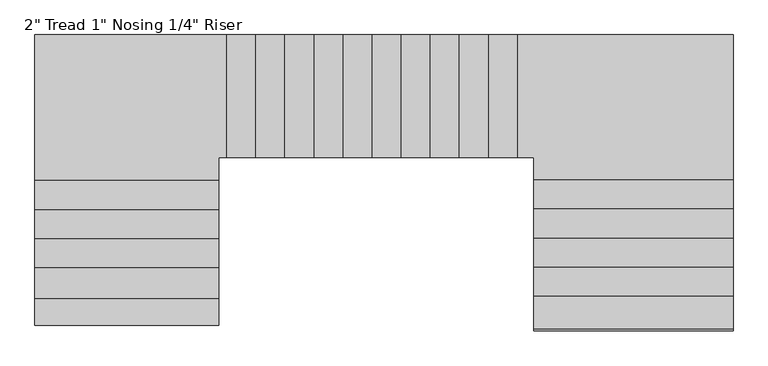
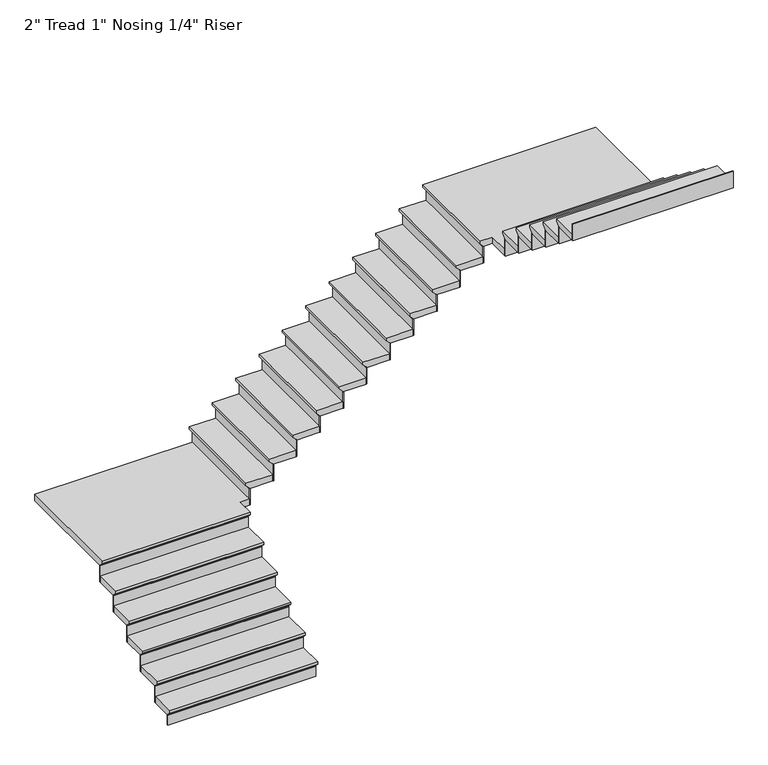
"""IFC4 building model written with IfcOpenShell, lengths in millimetres: stair flight geometry."""

from ifc_helpers import new_model, si_unit, origin, place, context, project, spatial, faceted_brep, source, transform, mapped, element, save


def stair_flight_3cceab32(model_context):
    return source(origin(), model_context, "Body", "Brep", [
        faceted_brep([(-2368.6972892, 4718.9167606, 6514.2717391), (-2368.6972892, 4718.9167606, 6533.3217391), (-3493.0046642, 4718.9167606, 6533.3217391), (-3493.0046642, 4718.9167606, 6514.2717391), (-2368.6972892, 4744.3167606, 6488.8717391), (-3493.0046642, 4744.3167606, 6488.8717391), (-2368.6972892, 4909.4167606, 6533.3217391), (-3493.0046642, 4909.4167606, 6533.3217391), (-3493.0046642, 4744.3167606, 6482.5217391), (-3493.0046642, 4909.4167606, 6482.5217391), (-2368.6972892, 4909.4167606, 6482.5217391), (-2368.6972892, 4744.3167606, 6482.5217391)], [[[0, 1, 2, 3]], [[4, 0, 3, 5]], [[2, 1, 6, 7]], [[8, 9, 10, 11]], [[2, 7, 9, 8, 5, 3]], [[8, 11, 4, 5]], [[6, 1, 0, 4, 11, 10]], [[7, 6, 10, 9]]]),
        faceted_brep([(-2368.6972892, 4744.3167606, 6482.5217391), (-2368.6972892, 4744.3167606, 6400.8), (-2368.6972892, 4750.6667606, 6400.8), (-2368.6972892, 4750.6667606, 6482.5217391), (-3493.0046642, 4744.3167606, 6482.5217391), (-3493.0046642, 4750.6667606, 6482.5217391), (-3493.0046642, 4750.6667606, 6400.8), (-3493.0046642, 4744.3167606, 6400.8)], [[[0, 1, 2, 3]], [[4, 5, 6, 7]], [[1, 0, 4, 7]], [[2, 1, 7, 6]], [[3, 2, 6, 5]], [[0, 3, 5, 4]]]),
        faceted_brep([(-2368.6972892, 4909.4167606, 6615.0434783), (-2368.6972892, 4909.4167606, 6482.5217391), (-2368.6972892, 4915.7667606, 6482.5217391), (-2368.6972892, 4915.7667606, 6615.0434783), (-3493.0046642, 4909.4167606, 6615.0434783), (-3493.0046642, 4915.7667606, 6615.0434783), (-3493.0046642, 4915.7667606, 6482.5217391), (-3493.0046642, 4909.4167606, 6482.5217391)], [[[0, 1, 2, 3]], [[4, 5, 6, 7]], [[1, 0, 4, 7]], [[2, 1, 7, 6]], [[3, 2, 6, 5]], [[0, 3, 5, 4]]]),
        faceted_brep([(-3493.0046642, 4884.0167606, 6665.8434783), (-2368.6972892, 4884.0167606, 6665.8434783), (-2368.6972892, 5099.9164494, 6665.8434783), (-3493.0046642, 5099.9164494, 6665.8434783), (-3493.0046642, 4909.4167606, 6615.0434783), (-3493.0046642, 5099.9164494, 6615.0434783), (-2368.6972892, 5099.9164494, 6615.0434783), (-2368.6972892, 4909.4167606, 6615.0434783), (-3493.0046642, 4909.4167606, 6621.3934783), (-3493.0046642, 4884.0167606, 6646.7934783), (-2368.6972892, 4909.4167606, 6621.3934783), (-2368.6972892, 4884.0167606, 6646.7934783)], [[[0, 1, 2, 3]], [[4, 5, 6, 7]], [[0, 3, 5, 4, 8, 9]], [[4, 7, 10, 8]], [[2, 1, 11, 10, 7, 6]], [[3, 2, 6, 5]], [[11, 1, 0, 9]], [[10, 11, 9, 8]]]),
        faceted_brep([(-2368.6972892, 5099.9164494, 6747.5652174), (-2368.6972892, 5099.9164494, 6615.0434783), (-2368.6972892, 5106.2664494, 6615.0434783), (-2368.6972892, 5106.2664494, 6747.5652174), (-3493.0046642, 5099.9164494, 6747.5652174), (-3493.0046642, 5106.2664494, 6747.5652174), (-3493.0046642, 5106.2664494, 6615.0434783), (-3493.0046642, 5099.9164494, 6615.0434783)], [[[0, 1, 2, 3]], [[4, 5, 6, 7]], [[1, 0, 4, 7]], [[2, 1, 7, 6]], [[3, 2, 6, 5]], [[0, 3, 5, 4]]]),
        faceted_brep([(-3493.0046642, 5074.5164494, 6798.3652174), (-2368.6972892, 5074.5164494, 6798.3652174), (-2368.6972892, 5277.7164494, 6798.3652174), (-3493.0046642, 5277.7164494, 6798.3652174), (-3493.0046642, 5099.9164494, 6747.5652174), (-3493.0046642, 5277.7164494, 6747.5652174), (-2368.6972892, 5277.7164494, 6747.5652174), (-2368.6972892, 5099.9164494, 6747.5652174), (-3493.0046642, 5099.9164494, 6753.9152174), (-3493.0046642, 5074.5164494, 6779.3152174), (-2368.6972892, 5099.9164494, 6753.9152174), (-2368.6972892, 5074.5164494, 6779.3152174)], [[[0, 1, 2, 3]], [[4, 5, 6, 7]], [[0, 3, 5, 4, 8, 9]], [[4, 7, 10, 8]], [[2, 1, 11, 10, 7, 6]], [[3, 2, 6, 5]], [[11, 1, 0, 9]], [[10, 11, 9, 8]]]),
        faceted_brep([(-2368.6972892, 5277.7164494, 6880.0869565), (-2368.6972892, 5277.7164494, 6747.5652174), (-2368.6972892, 5284.0664494, 6747.5652174), (-2368.6972892, 5284.0664494, 6880.0869565), (-3493.0046642, 5277.7164494, 6880.0869565), (-3493.0046642, 5284.0664494, 6880.0869565), (-3493.0046642, 5284.0664494, 6747.5652174), (-3493.0046642, 5277.7164494, 6747.5652174)], [[[0, 1, 2, 3]], [[4, 5, 6, 7]], [[1, 0, 4, 7]], [[2, 1, 7, 6]], [[3, 2, 6, 5]], [[0, 3, 5, 4]]]),
        faceted_brep([(-3493.0046642, 5252.3164494, 6930.8869565), (-2368.6972892, 5252.3164494, 6930.8869565), (-2368.6972892, 5455.5164494, 6930.8869565), (-3493.0046642, 5455.5164494, 6930.8869565), (-3493.0046642, 5277.7164494, 6880.0869565), (-3493.0046642, 5455.5164494, 6880.0869565), (-2368.6972892, 5455.5164494, 6880.0869565), (-2368.6972892, 5277.7164494, 6880.0869565), (-3493.0046642, 5277.7164494, 6886.4369565), (-3493.0046642, 5252.3164494, 6911.8369565), (-2368.6972892, 5277.7164494, 6886.4369565), (-2368.6972892, 5252.3164494, 6911.8369565)], [[[0, 1, 2, 3]], [[4, 5, 6, 7]], [[0, 3, 5, 4, 8, 9]], [[4, 7, 10, 8]], [[2, 1, 11, 10, 7, 6]], [[3, 2, 6, 5]], [[11, 1, 0, 9]], [[10, 11, 9, 8]]]),
        faceted_brep([(-2368.6972892, 5455.5164494, 7012.6086957), (-2368.6972892, 5455.5164494, 6880.0869565), (-2368.6972892, 5461.8664494, 6880.0869565), (-2368.6972892, 5461.8664494, 7012.6086957), (-3493.0046642, 5455.5164494, 7012.6086957), (-3493.0046642, 5461.8664494, 7012.6086957), (-3493.0046642, 5461.8664494, 6880.0869565), (-3493.0046642, 5455.5164494, 6880.0869565)], [[[0, 1, 2, 3]], [[4, 5, 6, 7]], [[1, 0, 4, 7]], [[2, 1, 7, 6]], [[3, 2, 6, 5]], [[0, 3, 5, 4]]]),
        faceted_brep([(-3493.0046642, 5430.1164494, 7063.4086957), (-2368.6972892, 5430.1164494, 7063.4086957), (-2368.6972892, 5633.3167606, 7063.4086957), (-3493.0046642, 5633.3167606, 7063.4086957), (-3493.0046642, 5455.5164494, 7012.6086957), (-3493.0046642, 5633.3167606, 7012.6086957), (-2368.6972892, 5633.3167606, 7012.6086957), (-2368.6972892, 5455.5164494, 7012.6086957), (-3493.0046642, 5455.5164494, 7018.9586957), (-3493.0046642, 5430.1164494, 7044.3586957), (-2368.6972892, 5455.5164494, 7018.9586957), (-2368.6972892, 5430.1164494, 7044.3586957)], [[[0, 1, 2, 3]], [[4, 5, 6, 7]], [[0, 3, 5, 4, 8, 9]], [[4, 7, 10, 8]], [[2, 1, 11, 10, 7, 6]], [[3, 2, 6, 5]], [[11, 1, 0, 9]], [[10, 11, 9, 8]]]),
        faceted_brep([(-2368.6972892, 5633.3167606, 7145.1304348), (-2368.6972892, 5633.3167606, 7012.6086957), (-2368.6972892, 5639.6667606, 7012.6086957), (-2368.6972892, 5639.6667606, 7145.1304348), (-3493.0046642, 5633.3167606, 7145.1304348), (-3493.0046642, 5639.6667606, 7145.1304348), (-3493.0046642, 5639.6667606, 7012.6086957), (-3493.0046642, 5633.3167606, 7012.6086957)], [[[0, 1, 2, 3]], [[4, 5, 6, 7]], [[1, 0, 4, 7]], [[2, 1, 7, 6]], [[3, 2, 6, 5]], [[0, 3, 5, 4]]]),
        faceted_brep([(-2295.032382, 6496.9167606, 7195.9304348), (-3493.0046642, 6496.9167606, 7195.9304348), (-3493.0046642, 5607.9167606, 7195.9304348), (-2368.6972892, 5607.9167606, 7195.9304348), (-2368.6972892, 5746.5536537, 7195.9304348), (-2295.032382, 5746.5536537, 7195.9304348), (-3493.0046642, 6496.9167606, 7145.1304348), (-2295.032382, 6496.9167606, 7145.1304348), (-2295.032382, 5746.5536537, 7145.1304348), (-2368.6972892, 5746.5536537, 7145.1304348), (-2368.6972892, 5633.3167606, 7145.1304348), (-3493.0046642, 5633.3167606, 7145.1304348), (-3493.0046642, 5633.3167606, 7151.4804348), (-3493.0046642, 5607.9167606, 7176.8804348), (-2368.6972892, 5633.3167606, 7151.4804348), (-2368.6972892, 5607.9167606, 7176.8804348)], [[[0, 1, 2, 3, 4, 5]], [[6, 7, 8, 9, 10, 11]], [[1, 0, 7, 6]], [[2, 1, 6, 11, 12, 13]], [[11, 10, 14, 12]], [[4, 3, 15, 14, 10, 9]], [[5, 4, 9, 8]], [[0, 5, 8, 7]], [[15, 3, 2, 13]], [[14, 15, 13, 12]]]),
        faceted_brep([(-2295.032382, 5746.5536537, 7277.6521739), (-2295.032382, 5746.5536537, 7145.1304348), (-2288.682382, 5746.5536537, 7145.1304348), (-2288.682382, 5746.5536537, 7277.6521739), (-2295.032382, 6496.9167606, 7277.6521739), (-2288.682382, 6496.9167606, 7277.6521739), (-2288.682382, 6496.9167606, 7145.1304348), (-2295.032382, 6496.9167606, 7145.1304348)], [[[0, 1, 2, 3]], [[4, 5, 6, 7]], [[1, 0, 4, 7]], [[2, 1, 7, 6]], [[3, 2, 6, 5]], [[0, 3, 5, 4]]]),
        faceted_brep([(-2320.432382, 6496.9167606, 7328.4521739), (-2320.432382, 5746.5536537, 7328.4521739), (-2117.232382, 5746.5536537, 7328.4521739), (-2117.232382, 6496.9167606, 7328.4521739), (-2295.032382, 6496.9167606, 7277.6521739), (-2117.232382, 6496.9167606, 7277.6521739), (-2117.232382, 5746.5536537, 7277.6521739), (-2295.032382, 5746.5536537, 7277.6521739), (-2295.032382, 6496.9167606, 7284.0021739), (-2320.432382, 6496.9167606, 7309.4021739), (-2295.032382, 5746.5536537, 7284.0021739), (-2320.432382, 5746.5536537, 7309.4021739)], [[[0, 1, 2, 3]], [[4, 5, 6, 7]], [[0, 3, 5, 4, 8, 9]], [[4, 7, 10, 8]], [[2, 1, 11, 10, 7, 6]], [[3, 2, 6, 5]], [[11, 1, 0, 9]], [[10, 11, 9, 8]]]),
        faceted_brep([(-2117.232382, 5746.5536537, 7410.173913), (-2117.232382, 5746.5536537, 7277.6521739), (-2110.882382, 5746.5536537, 7277.6521739), (-2110.882382, 5746.5536537, 7410.173913), (-2117.232382, 6496.9167606, 7410.173913), (-2110.882382, 6496.9167606, 7410.173913), (-2110.882382, 6496.9167606, 7277.6521739), (-2117.232382, 6496.9167606, 7277.6521739)], [[[0, 1, 2, 3]], [[4, 5, 6, 7]], [[1, 0, 4, 7]], [[2, 1, 7, 6]], [[3, 2, 6, 5]], [[0, 3, 5, 4]]]),
        faceted_brep([(-2142.632382, 6496.9167606, 7460.973913), (-2142.632382, 5746.5536537, 7460.973913), (-1939.432382, 5746.5536537, 7460.973913), (-1939.432382, 6496.9167606, 7460.973913), (-2117.232382, 6496.9167606, 7410.173913), (-1939.432382, 6496.9167606, 7410.173913), (-1939.432382, 5746.5536537, 7410.173913), (-2117.232382, 5746.5536537, 7410.173913), (-2117.232382, 6496.9167606, 7416.523913), (-2142.632382, 6496.9167606, 7441.923913), (-2117.232382, 5746.5536537, 7416.523913), (-2142.632382, 5746.5536537, 7441.923913)], [[[0, 1, 2, 3]], [[4, 5, 6, 7]], [[0, 3, 5, 4, 8, 9]], [[4, 7, 10, 8]], [[2, 1, 11, 10, 7, 6]], [[3, 2, 6, 5]], [[11, 1, 0, 9]], [[10, 11, 9, 8]]]),
        faceted_brep([(-1939.432382, 5746.5536537, 7542.6956522), (-1939.432382, 5746.5536537, 7410.173913), (-1933.082382, 5746.5536537, 7410.173913), (-1933.082382, 5746.5536537, 7542.6956522), (-1939.432382, 6496.9167606, 7542.6956522), (-1933.082382, 6496.9167606, 7542.6956522), (-1933.082382, 6496.9167606, 7410.173913), (-1939.432382, 6496.9167606, 7410.173913)], [[[0, 1, 2, 3]], [[4, 5, 6, 7]], [[1, 0, 4, 7]], [[2, 1, 7, 6]], [[3, 2, 6, 5]], [[0, 3, 5, 4]]]),
        faceted_brep([(-1964.832382, 6496.9167606, 7593.4956522), (-1964.832382, 5746.5536537, 7593.4956522), (-1761.632382, 5746.5536537, 7593.4956522), (-1761.632382, 6496.9167606, 7593.4956522), (-1939.432382, 6496.9167606, 7542.6956522), (-1761.632382, 6496.9167606, 7542.6956522), (-1761.632382, 5746.5536537, 7542.6956522), (-1939.432382, 5746.5536537, 7542.6956522), (-1939.432382, 6496.9167606, 7549.0456522), (-1964.832382, 6496.9167606, 7574.4456522), (-1939.432382, 5746.5536537, 7549.0456522), (-1964.832382, 5746.5536537, 7574.4456522)], [[[0, 1, 2, 3]], [[4, 5, 6, 7]], [[0, 3, 5, 4, 8, 9]], [[4, 7, 10, 8]], [[2, 1, 11, 10, 7, 6]], [[3, 2, 6, 5]], [[11, 1, 0, 9]], [[10, 11, 9, 8]]]),
        faceted_brep([(-1761.632382, 5746.5536537, 7675.2173913), (-1761.632382, 5746.5536537, 7542.6956522), (-1755.282382, 5746.5536537, 7542.6956522), (-1755.282382, 5746.5536537, 7675.2173913), (-1761.632382, 6496.9167606, 7675.2173913), (-1755.282382, 6496.9167606, 7675.2173913), (-1755.282382, 6496.9167606, 7542.6956522), (-1761.632382, 6496.9167606, 7542.6956522)], [[[0, 1, 2, 3]], [[4, 5, 6, 7]], [[1, 0, 4, 7]], [[2, 1, 7, 6]], [[3, 2, 6, 5]], [[0, 3, 5, 4]]]),
        faceted_brep([(-1787.032382, 6496.9167606, 7726.0173913), (-1787.032382, 5746.5536537, 7726.0173913), (-1583.832382, 5746.5536537, 7726.0173913), (-1583.832382, 6496.9167606, 7726.0173913), (-1761.632382, 6496.9167606, 7675.2173913), (-1583.832382, 6496.9167606, 7675.2173913), (-1583.832382, 5746.5536537, 7675.2173913), (-1761.632382, 5746.5536537, 7675.2173913), (-1761.632382, 6496.9167606, 7681.5673913), (-1787.032382, 6496.9167606, 7706.9673913), (-1761.632382, 5746.5536537, 7681.5673913), (-1787.032382, 5746.5536537, 7706.9673913)], [[[0, 1, 2, 3]], [[4, 5, 6, 7]], [[0, 3, 5, 4, 8, 9]], [[4, 7, 10, 8]], [[2, 1, 11, 10, 7, 6]], [[3, 2, 6, 5]], [[11, 1, 0, 9]], [[10, 11, 9, 8]]]),
        faceted_brep([(-1583.832382, 5746.5536537, 7807.7391304), (-1583.832382, 5746.5536537, 7675.2173913), (-1577.482382, 5746.5536537, 7675.2173913), (-1577.482382, 5746.5536537, 7807.7391304), (-1583.832382, 6496.9167606, 7807.7391304), (-1577.482382, 6496.9167606, 7807.7391304), (-1577.482382, 6496.9167606, 7675.2173913), (-1583.832382, 6496.9167606, 7675.2173913)], [[[0, 1, 2, 3]], [[4, 5, 6, 7]], [[1, 0, 4, 7]], [[2, 1, 7, 6]], [[3, 2, 6, 5]], [[0, 3, 5, 4]]]),
        faceted_brep([(-1609.232382, 6496.9167606, 7858.5391304), (-1609.232382, 5746.5536537, 7858.5391304), (-1406.032382, 5746.5536537, 7858.5391304), (-1406.032382, 6496.9167606, 7858.5391304), (-1583.832382, 6496.9167606, 7807.7391304), (-1406.032382, 6496.9167606, 7807.7391304), (-1406.032382, 5746.5536537, 7807.7391304), (-1583.832382, 5746.5536537, 7807.7391304), (-1583.832382, 6496.9167606, 7814.0891304), (-1609.232382, 6496.9167606, 7839.4891304), (-1583.832382, 5746.5536537, 7814.0891304), (-1609.232382, 5746.5536537, 7839.4891304)], [[[0, 1, 2, 3]], [[4, 5, 6, 7]], [[0, 3, 5, 4, 8, 9]], [[4, 7, 10, 8]], [[2, 1, 11, 10, 7, 6]], [[3, 2, 6, 5]], [[11, 1, 0, 9]], [[10, 11, 9, 8]]]),
        faceted_brep([(-1406.032382, 5746.5536537, 7940.2608696), (-1406.032382, 5746.5536537, 7807.7391304), (-1399.682382, 5746.5536537, 7807.7391304), (-1399.682382, 5746.5536537, 7940.2608696), (-1406.032382, 6496.9167606, 7940.2608696), (-1399.682382, 6496.9167606, 7940.2608696), (-1399.682382, 6496.9167606, 7807.7391304), (-1406.032382, 6496.9167606, 7807.7391304)], [[[0, 1, 2, 3]], [[4, 5, 6, 7]], [[1, 0, 4, 7]], [[2, 1, 7, 6]], [[3, 2, 6, 5]], [[0, 3, 5, 4]]]),
        faceted_brep([(-1431.432382, 6496.9167606, 7991.0608696), (-1431.432382, 5746.5536537, 7991.0608696), (-1228.232382, 5746.5536537, 7991.0608696), (-1228.232382, 6496.9167606, 7991.0608696), (-1406.032382, 6496.9167606, 7940.2608696), (-1228.232382, 6496.9167606, 7940.2608696), (-1228.232382, 5746.5536537, 7940.2608696), (-1406.032382, 5746.5536537, 7940.2608696), (-1406.032382, 6496.9167606, 7946.6108696), (-1431.432382, 6496.9167606, 7972.0108696), (-1406.032382, 5746.5536537, 7946.6108696), (-1431.432382, 5746.5536537, 7972.0108696)], [[[0, 1, 2, 3]], [[4, 5, 6, 7]], [[0, 3, 5, 4, 8, 9]], [[4, 7, 10, 8]], [[2, 1, 11, 10, 7, 6]], [[3, 2, 6, 5]], [[11, 1, 0, 9]], [[10, 11, 9, 8]]]),
        faceted_brep([(-1228.232382, 5746.5536537, 8072.7826087), (-1228.232382, 5746.5536537, 7940.2608696), (-1221.882382, 5746.5536537, 7940.2608696), (-1221.882382, 5746.5536537, 8072.7826087), (-1228.232382, 6496.9167606, 8072.7826087), (-1221.882382, 6496.9167606, 8072.7826087), (-1221.882382, 6496.9167606, 7940.2608696), (-1228.232382, 6496.9167606, 7940.2608696)], [[[0, 1, 2, 3]], [[4, 5, 6, 7]], [[1, 0, 4, 7]], [[2, 1, 7, 6]], [[3, 2, 6, 5]], [[0, 3, 5, 4]]]),
        faceted_brep([(-1253.632382, 6496.9167606, 8123.5826087), (-1253.632382, 5746.5536537, 8123.5826087), (-1050.432382, 5746.5536537, 8123.5826087), (-1050.432382, 6496.9167606, 8123.5826087), (-1228.232382, 6496.9167606, 8072.7826087), (-1050.432382, 6496.9167606, 8072.7826087), (-1050.432382, 5746.5536537, 8072.7826087), (-1228.232382, 5746.5536537, 8072.7826087), (-1228.232382, 6496.9167606, 8079.1326087), (-1253.632382, 6496.9167606, 8104.5326087), (-1228.232382, 5746.5536537, 8079.1326087), (-1253.632382, 5746.5536537, 8104.5326087)], [[[0, 1, 2, 3]], [[4, 5, 6, 7]], [[0, 3, 5, 4, 8, 9]], [[4, 7, 10, 8]], [[2, 1, 11, 10, 7, 6]], [[3, 2, 6, 5]], [[11, 1, 0, 9]], [[10, 11, 9, 8]]]),
        faceted_brep([(-1050.432382, 5746.5536537, 8205.3043478), (-1050.432382, 5746.5536537, 8072.7826087), (-1044.082382, 5746.5536537, 8072.7826087), (-1044.082382, 5746.5536537, 8205.3043478), (-1050.432382, 6496.9167606, 8205.3043478), (-1044.082382, 6496.9167606, 8205.3043478), (-1044.082382, 6496.9167606, 8072.7826087), (-1050.432382, 6496.9167606, 8072.7826087)], [[[0, 1, 2, 3]], [[4, 5, 6, 7]], [[1, 0, 4, 7]], [[2, 1, 7, 6]], [[3, 2, 6, 5]], [[0, 3, 5, 4]]]),
        faceted_brep([(-1075.832382, 6496.9167606, 8256.1043478), (-1075.832382, 5746.5536537, 8256.1043478), (-872.632382, 5746.5536537, 8256.1043478), (-872.632382, 6496.9167606, 8256.1043478), (-1050.432382, 6496.9167606, 8205.3043478), (-872.632382, 6496.9167606, 8205.3043478), (-872.632382, 5746.5536537, 8205.3043478), (-1050.432382, 5746.5536537, 8205.3043478), (-1050.432382, 6496.9167606, 8211.6543478), (-1075.832382, 6496.9167606, 8237.0543478), (-1050.432382, 5746.5536537, 8211.6543478), (-1075.832382, 5746.5536537, 8237.0543478)], [[[0, 1, 2, 3]], [[4, 5, 6, 7]], [[0, 3, 5, 4, 8, 9]], [[4, 7, 10, 8]], [[2, 1, 11, 10, 7, 6]], [[3, 2, 6, 5]], [[11, 1, 0, 9]], [[10, 11, 9, 8]]]),
        faceted_brep([(-872.632382, 5746.5536537, 8337.826087), (-872.632382, 5746.5536537, 8205.3043478), (-866.282382, 5746.5536537, 8205.3043478), (-866.282382, 5746.5536537, 8337.826087), (-872.632382, 6496.9167606, 8337.826087), (-866.282382, 6496.9167606, 8337.826087), (-866.282382, 6496.9167606, 8205.3043478), (-872.632382, 6496.9167606, 8205.3043478)], [[[0, 1, 2, 3]], [[4, 5, 6, 7]], [[1, 0, 4, 7]], [[2, 1, 7, 6]], [[3, 2, 6, 5]], [[0, 3, 5, 4]]]),
        faceted_brep([(-898.032382, 6496.9167606, 8388.626087), (-898.032382, 5746.5536537, 8388.626087), (-694.832382, 5746.5536537, 8388.626087), (-694.832382, 6496.9167606, 8388.626087), (-872.632382, 6496.9167606, 8337.826087), (-694.832382, 6496.9167606, 8337.826087), (-694.832382, 5746.5536537, 8337.826087), (-872.632382, 5746.5536537, 8337.826087), (-872.632382, 6496.9167606, 8344.176087), (-898.032382, 6496.9167606, 8369.576087), (-872.632382, 5746.5536537, 8344.176087), (-898.032382, 5746.5536537, 8369.576087)], [[[0, 1, 2, 3]], [[4, 5, 6, 7]], [[0, 3, 5, 4, 8, 9]], [[4, 7, 10, 8]], [[2, 1, 11, 10, 7, 6]], [[3, 2, 6, 5]], [[11, 1, 0, 9]], [[10, 11, 9, 8]]]),
        faceted_brep([(-694.832382, 5746.5536537, 8470.3478261), (-694.832382, 5746.5536537, 8337.826087), (-688.482382, 5746.5536537, 8337.826087), (-688.482382, 5746.5536537, 8470.3478261), (-694.832382, 6496.9167606, 8470.3478261), (-688.482382, 6496.9167606, 8470.3478261), (-688.482382, 6496.9167606, 8337.826087), (-694.832382, 6496.9167606, 8337.826087)], [[[0, 1, 2, 3]], [[4, 5, 6, 7]], [[1, 0, 4, 7]], [[2, 1, 7, 6]], [[3, 2, 6, 5]], [[0, 3, 5, 4]]]),
        faceted_brep([(-720.232382, 6496.9167606, 8521.1478261), (-720.232382, 5746.5536537, 8521.1478261), (-517.032382, 5746.5536537, 8521.1478261), (-517.032382, 6496.9167606, 8521.1478261), (-694.832382, 6496.9167606, 8470.3478261), (-517.032382, 6496.9167606, 8470.3478261), (-517.032382, 5746.5536537, 8470.3478261), (-694.832382, 5746.5536537, 8470.3478261), (-694.832382, 6496.9167606, 8476.6978261), (-720.232382, 6496.9167606, 8502.0978261), (-694.832382, 5746.5536537, 8476.6978261), (-720.232382, 5746.5536537, 8502.0978261)], [[[0, 1, 2, 3]], [[4, 5, 6, 7]], [[0, 3, 5, 4, 8, 9]], [[4, 7, 10, 8]], [[2, 1, 11, 10, 7, 6]], [[3, 2, 6, 5]], [[11, 1, 0, 9]], [[10, 11, 9, 8]]]),
        faceted_brep([(-517.032382, 5746.5536537, 8602.8695652), (-517.032382, 5746.5536537, 8470.3478261), (-510.682382, 5746.5536537, 8470.3478261), (-510.682382, 5746.5536537, 8602.8695652), (-517.032382, 6496.9167606, 8602.8695652), (-510.682382, 6496.9167606, 8602.8695652), (-510.682382, 6496.9167606, 8470.3478261), (-517.032382, 6496.9167606, 8470.3478261)], [[[0, 1, 2, 3]], [[4, 5, 6, 7]], [[1, 0, 4, 7]], [[2, 1, 7, 6]], [[3, 2, 6, 5]], [[0, 3, 5, 4]]]),
        faceted_brep([(774.1953358, 5582.5167606, 8653.6695652), (774.1953358, 6496.9167606, 8653.6695652), (-542.432382, 6496.9167606, 8653.6695652), (-542.432382, 5746.5536537, 8653.6695652), (-445.0046642, 5746.5536537, 8653.6695652), (-445.0046642, 5582.5167606, 8653.6695652), (774.1953358, 6496.9167606, 8602.8695652), (774.1953358, 5582.5167606, 8602.8695652), (-445.0046642, 5582.5167606, 8602.8695652), (-445.0046642, 5746.5536537, 8602.8695652), (-517.032382, 5746.5536537, 8602.8695652), (-517.032382, 6496.9167606, 8602.8695652), (-517.032382, 6496.9167606, 8609.2195652), (-542.432382, 6496.9167606, 8634.6195652), (-517.032382, 5746.5536537, 8609.2195652), (-542.432382, 5746.5536537, 8634.6195652)], [[[0, 1, 2, 3, 4, 5]], [[6, 7, 8, 9, 10, 11]], [[1, 0, 7, 6]], [[2, 1, 6, 11, 12, 13]], [[11, 10, 14, 12]], [[4, 3, 15, 14, 10, 9]], [[5, 4, 9, 8]], [[0, 5, 8, 7]], [[15, 3, 2, 13]], [[14, 15, 13, 12]]]),
        faceted_brep([(-445.0046642, 5582.5167606, 8735.3913043), (-445.0046642, 5582.5167606, 8602.8695652), (-445.0046642, 5576.1667606, 8602.8695652), (-445.0046642, 5576.1667606, 8735.3913043), (774.1953358, 5582.5167606, 8735.3913043), (774.1953358, 5576.1667606, 8735.3913043), (774.1953358, 5576.1667606, 8602.8695652), (774.1953358, 5582.5167606, 8602.8695652)], [[[0, 1, 2, 3]], [[4, 5, 6, 7]], [[1, 0, 4, 7]], [[2, 1, 7, 6]], [[3, 2, 6, 5]], [[0, 3, 5, 4]]]),
        faceted_brep([(774.1953358, 5607.9167606, 8786.1913043), (-445.0046642, 5607.9167606, 8786.1913043), (-445.0046642, 5404.7164494, 8786.1913043), (774.1953358, 5404.7164494, 8786.1913043), (774.1953358, 5582.5167606, 8735.3913043), (774.1953358, 5404.7164494, 8735.3913043), (-445.0046642, 5404.7164494, 8735.3913043), (-445.0046642, 5582.5167606, 8735.3913043), (774.1953358, 5582.5167606, 8741.7413043), (774.1953358, 5607.9167606, 8767.1413043), (-445.0046642, 5582.5167606, 8741.7413043), (-445.0046642, 5607.9167606, 8767.1413043)], [[[0, 1, 2, 3]], [[4, 5, 6, 7]], [[0, 3, 5, 4, 8, 9]], [[4, 7, 10, 8]], [[2, 1, 11, 10, 7, 6]], [[3, 2, 6, 5]], [[11, 1, 0, 9]], [[10, 11, 9, 8]]]),
        faceted_brep([(-445.0046642, 5404.7164494, 8867.9130435), (-445.0046642, 5404.7164494, 8735.3913043), (-445.0046642, 5398.3664494, 8735.3913043), (-445.0046642, 5398.3664494, 8867.9130435), (774.1953358, 5404.7164494, 8867.9130435), (774.1953358, 5398.3664494, 8867.9130435), (774.1953358, 5398.3664494, 8735.3913043), (774.1953358, 5404.7164494, 8735.3913043)], [[[0, 1, 2, 3]], [[4, 5, 6, 7]], [[1, 0, 4, 7]], [[2, 1, 7, 6]], [[3, 2, 6, 5]], [[0, 3, 5, 4]]]),
        faceted_brep([(774.1953358, 5430.1164494, 8918.7130435), (-445.0046642, 5430.1164494, 8918.7130435), (-445.0046642, 5226.9164494, 8918.7130435), (774.1953358, 5226.9164494, 8918.7130435), (774.1953358, 5404.7164494, 8867.9130435), (774.1953358, 5226.9164494, 8867.9130435), (-445.0046642, 5226.9164494, 8867.9130435), (-445.0046642, 5404.7164494, 8867.9130435), (774.1953358, 5404.7164494, 8874.2630435), (774.1953358, 5430.1164494, 8899.6630435), (-445.0046642, 5404.7164494, 8874.2630435), (-445.0046642, 5430.1164494, 8899.6630435)], [[[0, 1, 2, 3]], [[4, 5, 6, 7]], [[0, 3, 5, 4, 8, 9]], [[4, 7, 10, 8]], [[2, 1, 11, 10, 7, 6]], [[3, 2, 6, 5]], [[11, 1, 0, 9]], [[10, 11, 9, 8]]]),
        faceted_brep([(-445.0046642, 5226.9164494, 9000.4347826), (-445.0046642, 5226.9164494, 8867.9130435), (-445.0046642, 5220.5664494, 8867.9130435), (-445.0046642, 5220.5664494, 9000.4347826), (774.1953358, 5226.9164494, 9000.4347826), (774.1953358, 5220.5664494, 9000.4347826), (774.1953358, 5220.5664494, 8867.9130435), (774.1953358, 5226.9164494, 8867.9130435)], [[[0, 1, 2, 3]], [[4, 5, 6, 7]], [[1, 0, 4, 7]], [[2, 1, 7, 6]], [[3, 2, 6, 5]], [[0, 3, 5, 4]]]),
        faceted_brep([(774.1953358, 5252.3164494, 9051.2347826), (-445.0046642, 5252.3164494, 9051.2347826), (-445.0046642, 5049.1164494, 9051.2347826), (774.1953358, 5049.1164494, 9051.2347826), (774.1953358, 5226.9164494, 9000.4347826), (774.1953358, 5049.1164494, 9000.4347826), (-445.0046642, 5049.1164494, 9000.4347826), (-445.0046642, 5226.9164494, 9000.4347826), (774.1953358, 5226.9164494, 9006.7847826), (774.1953358, 5252.3164494, 9032.1847826), (-445.0046642, 5226.9164494, 9006.7847826), (-445.0046642, 5252.3164494, 9032.1847826)], [[[0, 1, 2, 3]], [[4, 5, 6, 7]], [[0, 3, 5, 4, 8, 9]], [[4, 7, 10, 8]], [[2, 1, 11, 10, 7, 6]], [[3, 2, 6, 5]], [[11, 1, 0, 9]], [[10, 11, 9, 8]]]),
        faceted_brep([(-445.0046642, 5049.1164494, 9132.9565217), (-445.0046642, 5049.1164494, 9000.4347826), (-445.0046642, 5042.7664494, 9000.4347826), (-445.0046642, 5042.7664494, 9132.9565217), (774.1953358, 5049.1164494, 9132.9565217), (774.1953358, 5042.7664494, 9132.9565217), (774.1953358, 5042.7664494, 9000.4347826), (774.1953358, 5049.1164494, 9000.4347826)], [[[0, 1, 2, 3]], [[4, 5, 6, 7]], [[1, 0, 4, 7]], [[2, 1, 7, 6]], [[3, 2, 6, 5]], [[0, 3, 5, 4]]]),
        faceted_brep([(774.1953358, 5074.5164494, 9183.7565217), (-445.0046642, 5074.5164494, 9183.7565217), (-445.0046642, 4871.3164494, 9183.7565217), (774.1953358, 4871.3164494, 9183.7565217), (774.1953358, 5049.1164494, 9132.9565217), (774.1953358, 4871.3164494, 9132.9565217), (-445.0046642, 4871.3164494, 9132.9565217), (-445.0046642, 5049.1164494, 9132.9565217), (774.1953358, 5049.1164494, 9139.3065217), (774.1953358, 5074.5164494, 9164.7065217), (-445.0046642, 5049.1164494, 9139.3065217), (-445.0046642, 5074.5164494, 9164.7065217)], [[[0, 1, 2, 3]], [[4, 5, 6, 7]], [[0, 3, 5, 4, 8, 9]], [[4, 7, 10, 8]], [[2, 1, 11, 10, 7, 6]], [[3, 2, 6, 5]], [[11, 1, 0, 9]], [[10, 11, 9, 8]]]),
        faceted_brep([(-445.0046642, 4871.3164494, 9265.4782609), (-445.0046642, 4871.3164494, 9132.9565217), (-445.0046642, 4864.9664494, 9132.9565217), (-445.0046642, 4864.9664494, 9265.4782609), (774.1953358, 4871.3164494, 9265.4782609), (774.1953358, 4864.9664494, 9265.4782609), (774.1953358, 4864.9664494, 9132.9565217), (774.1953358, 4871.3164494, 9132.9565217)], [[[0, 1, 2, 3]], [[4, 5, 6, 7]], [[1, 0, 4, 7]], [[2, 1, 7, 6]], [[3, 2, 6, 5]], [[0, 3, 5, 4]]]),
        faceted_brep([(-445.0046642, 4693.5167606, 9398.0), (-445.0046642, 4693.5167606, 9265.4782609), (-445.0046642, 4687.1667606, 9265.4782609), (-445.0046642, 4687.1667606, 9398.0), (774.1953358, 4693.5167606, 9398.0), (774.1953358, 4687.1667606, 9398.0), (774.1953358, 4687.1667606, 9265.4782609), (774.1953358, 4693.5167606, 9265.4782609)], [[[0, 1, 2, 3]], [[4, 5, 6, 7]], [[1, 0, 4, 7]], [[2, 1, 7, 6]], [[3, 2, 6, 5]], [[0, 3, 5, 4]]]),
        faceted_brep([(774.1953358, 4896.7164494, 9316.2782609), (-445.0046642, 4896.7164494, 9316.2782609), (-445.0046642, 4693.5167606, 9316.2782609), (774.1953358, 4693.5167606, 9316.2782609), (774.1953358, 4871.3164494, 9265.4782609), (774.1953358, 4693.5167606, 9265.4782609), (-445.0046642, 4693.5167606, 9265.4782609), (-445.0046642, 4871.3164494, 9265.4782609), (774.1953358, 4871.3164494, 9271.8282609), (774.1953358, 4896.7164494, 9297.2282609), (-445.0046642, 4871.3164494, 9271.8282609), (-445.0046642, 4896.7164494, 9297.2282609)], [[[0, 1, 2, 3]], [[4, 5, 6, 7]], [[0, 3, 5, 4, 8, 9]], [[4, 7, 10, 8]], [[2, 1, 11, 10, 7, 6]], [[3, 2, 6, 5]], [[11, 1, 0, 9]], [[10, 11, 9, 8]]]),
    ])


if __name__ == "__main__":
    model = new_model("IFC4")
    model_context = context("Model", 3, world=origin())
    ifc_project = project(units=[si_unit("LENGTHUNIT", "METRE", prefix="MILLI")], contexts=[model_context])
    site = spatial("IfcSite", under=ifc_project)
    building = spatial("IfcBuilding", under=site)
    placement = place(None, origin())
    stair_flight_shape = stair_flight_3cceab32(model_context)
    element("IfcStairFlight", 1, ObjectType="2\" Tread 1\" Nosing 1/4\" Riser", at=placement, inside=building, context=model_context, shape_type="MappedRepresentation", body=[
        mapped(stair_flight_shape, transform((0.0, 0.0, 0.0), x_axis=(1.0, 0.0, 0.0), y_axis=(0.0, 1.0, 0.0), z_axis=(0.0, 0.0, 1.0))),
    ])
    save(model, "model.ifc")
